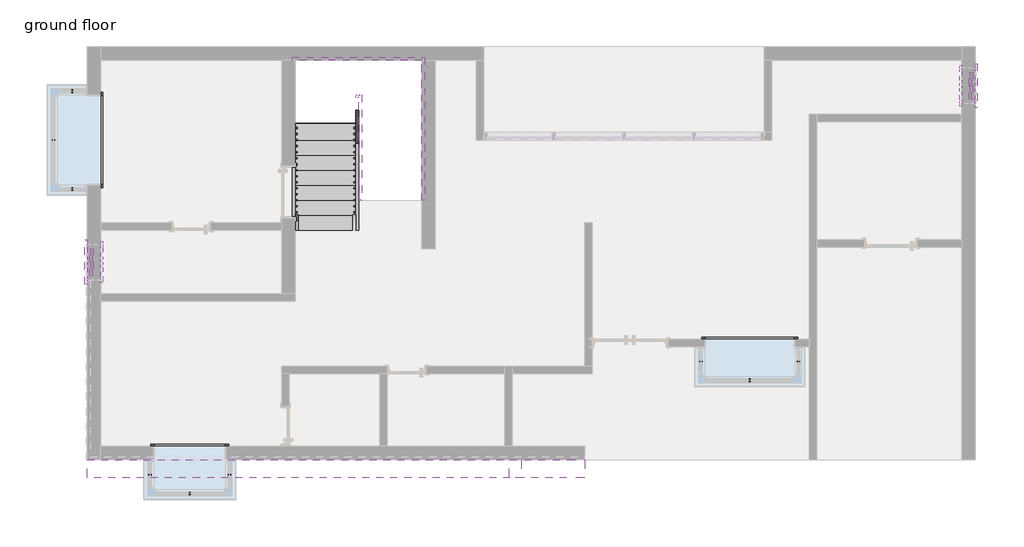
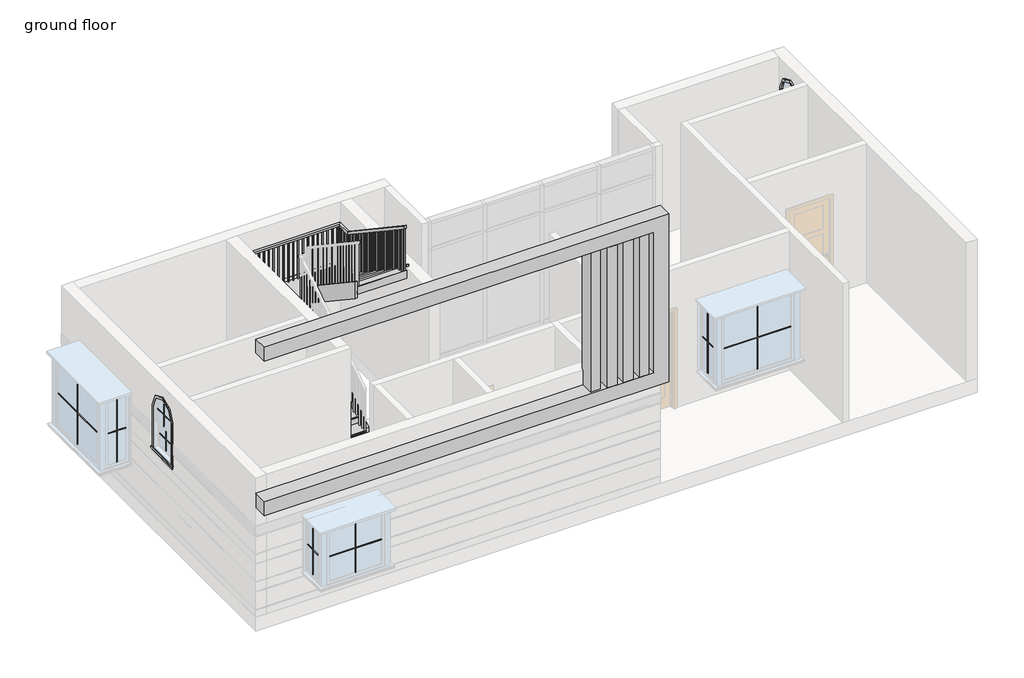
# One storey, part 5 of 5: 22 proxies, 6 members, 1 railing, 1 stair flight.
"""IFC4 building model written with IfcOpenShell, lengths in millimetres."""

from ifc_helpers import new_model, si_unit, frame, origin, place, context, project, spatial, polyline, outline, extrude, faceted_brep, transform, mapped, element, save
from components import generic_models_1_generic_models_1_e2d67b9d, generic_models_2_generic_models_2_13199aed, muntin_pattern_2x2_muntin_pattern_2x2_eeef18e2, muntin_pattern_2x2_muntin_pattern_2x2_218eda85, muntin_pattern_2x2_muntin_pattern_2x2_3440c8d2, muntin_pattern_2x2_muntin_pattern_2x2_8235f178, muntin_pattern_2x2_muntin_pattern_2x2_f03ab90d, trim_window_exterior_arch_hung_with_sill_ae9dfc94, trim_window_interior_arch_hung_picture_frame_76300bdb, trim_window_interior_flat_picture_frame_524b5c54, trim_window_interior_flat_picture_frame_ace0ae79, stair_flight_95751e6d

model = new_model("IFC4")

# Units and contexts
model_context = context("Model", 3, world=origin())
ifc_project = project(units=[si_unit("LENGTHUNIT", "METRE", prefix="MILLI")], contexts=[model_context])

# Site, building, storey
site = spatial("IfcSite", under=ifc_project)
building = spatial("IfcBuilding", under=site)
storey = spatial("IfcBuildingStorey", under=building, Name="ground floor", Elevation=304.8)

# Proxies
placement = place(None, origin())
generic_models_1_generic_models_1_shape = generic_models_1_generic_models_1_e2d67b9d(model_context)
element("IfcBuildingElementProxy", 1, Name="Generic Models 1 : Generic Models 1", ObjectType="Generic Models 1 : Generic Models 1", at=placement, inside=storey, context=model_context, shape_type="MappedRepresentation", body=[
    mapped(generic_models_1_generic_models_1_shape, transform((0.0, 0.0, 0.0), x_axis=(1.0, 0.0, 0.0), y_axis=(0.0, 1.0, 0.0), z_axis=(0.0, 0.0, 1.0))),
])
generic_models_2_generic_models_2_shape = generic_models_2_generic_models_2_13199aed(model_context)
element("IfcBuildingElementProxy", 2, Name="Generic Models 2 : Generic Models 2", ObjectType="Generic Models 2 : Generic Models 2", at=placement, inside=storey, context=model_context, shape_type="MappedRepresentation", body=[
    mapped(generic_models_2_generic_models_2_shape, transform((0.0, 0.0, 0.0), x_axis=(1.0, 0.0, 0.0), y_axis=(0.0, 1.0, 0.0), z_axis=(0.0, 0.0, 1.0))),
])
muntin_pattern_2x2_muntin_pattern_2x2_shape = muntin_pattern_2x2_muntin_pattern_2x2_eeef18e2(model_context)
element("IfcBuildingElementProxy", 3, Name="Muntin Pattern_2x2 : Muntin Pattern_2x2", ObjectType="Muntin Pattern_2x2 : Muntin Pattern_2x2", at=placement, inside=storey, context=model_context, shape_type="MappedRepresentation", body=[
    mapped(muntin_pattern_2x2_muntin_pattern_2x2_shape, transform((-2015.7672301, -5928.5552427, 1035.05), x_axis=(-1.0, 0.0, 0.0), y_axis=(0.0, -1.0, 0.0), z_axis=(0.0, 0.0, 1.0))),
])
element("IfcBuildingElementProxy", 4, Name="Muntin Pattern_2x2 : Muntin Pattern_2x2", ObjectType="Muntin Pattern_2x2 : Muntin Pattern_2x2", at=placement, inside=storey, context=model_context, shape_type="MappedRepresentation", body=[
    mapped(muntin_pattern_2x2_muntin_pattern_2x2_shape, transform((-13747.3922301, -1880.4302427, 1035.05), x_axis=(0.0, 1.0, 0.0), y_axis=(-1.0, 0.0, 0.0), z_axis=(0.0, 0.0, 1.0))),
])
muntin_pattern_2x2_muntin_pattern_2x2_2_shape = muntin_pattern_2x2_muntin_pattern_2x2_218eda85(model_context)
element("IfcBuildingElementProxy", 5, Name="Muntin Pattern_2x2 : Muntin Pattern_2x2", ObjectType="Muntin Pattern_2x2 : Muntin Pattern_2x2", at=placement, inside=storey, context=model_context, shape_type="MappedRepresentation", body=[
    mapped(muntin_pattern_2x2_muntin_pattern_2x2_2_shape, transform((-1193.4422301, -5614.2302427, 1035.05), x_axis=(0.0, 1.0, 0.0), y_axis=(-1.0, 0.0, 0.0), z_axis=(0.0, 0.0, 1.0))),
])
element("IfcBuildingElementProxy", 6, Name="Muntin Pattern_2x2 : Muntin Pattern_2x2", ObjectType="Muntin Pattern_2x2 : Muntin Pattern_2x2", at=placement, inside=storey, context=model_context, shape_type="MappedRepresentation", body=[
    mapped(muntin_pattern_2x2_muntin_pattern_2x2_2_shape, transform((-2838.0922301, -5614.2302427, 1035.05), x_axis=(0.0, -1.0, 0.0), y_axis=(1.0, 0.0, 0.0), z_axis=(0.0, 0.0, 1.0))),
])
element("IfcBuildingElementProxy", 7, Name="Muntin Pattern_2x2 : Muntin Pattern_2x2", ObjectType="Muntin Pattern_2x2 : Muntin Pattern_2x2", at=placement, inside=storey, context=model_context, shape_type="MappedRepresentation", body=[
    mapped(muntin_pattern_2x2_muntin_pattern_2x2_2_shape, transform((-13433.0672301, -2702.7552427, 1035.05), x_axis=(1.0, 0.0, 0.0), y_axis=(0.0, 1.0, 0.0), z_axis=(0.0, 0.0, 1.0))),
])
element("IfcBuildingElementProxy", 8, Name="Muntin Pattern_2x2 : Muntin Pattern_2x2", ObjectType="Muntin Pattern_2x2 : Muntin Pattern_2x2", at=placement, inside=storey, context=model_context, shape_type="MappedRepresentation", body=[
    mapped(muntin_pattern_2x2_muntin_pattern_2x2_2_shape, transform((-13433.0672301, -1058.1052427, 1035.05), x_axis=(-1.0, 0.0, 0.0), y_axis=(0.0, -1.0, 0.0), z_axis=(0.0, 0.0, 1.0))),
])
muntin_pattern_2x2_muntin_pattern_2x2_3_shape = muntin_pattern_2x2_muntin_pattern_2x2_3440c8d2(model_context)
element("IfcBuildingElementProxy", 9, Name="Muntin Pattern_2x2 : Muntin Pattern_2x2", ObjectType="Muntin Pattern_2x2 : Muntin Pattern_2x2", at=placement, inside=storey, context=model_context, shape_type="MappedRepresentation", body=[
    mapped(muntin_pattern_2x2_muntin_pattern_2x2_3_shape, transform((-13144.1422301, -3937.8302427, 2460.625), x_axis=(0.0, 1.0, 0.0), y_axis=(-1.0, 0.0, 0.0), z_axis=(0.0, 0.0, 1.0))),
])
element("IfcBuildingElementProxy", 10, Name="Muntin Pattern_2x2 : Muntin Pattern_2x2", ObjectType="Muntin Pattern_2x2 : Muntin Pattern_2x2", at=placement, inside=storey, context=model_context, shape_type="MappedRepresentation", body=[
    mapped(muntin_pattern_2x2_muntin_pattern_2x2_3_shape, transform((-13099.6922301, -3937.8302427, 1905.0), x_axis=(0.0, 1.0, 0.0), y_axis=(-1.0, 0.0, 0.0), z_axis=(0.0, 0.0, 1.0))),
])
element("IfcBuildingElementProxy", 11, Name="Muntin Pattern_2x2 : Muntin Pattern_2x2", ObjectType="Muntin Pattern_2x2 : Muntin Pattern_2x2", at=placement, inside=storey, context=model_context, shape_type="MappedRepresentation", body=[
    mapped(muntin_pattern_2x2_muntin_pattern_2x2_3_shape, transform((1746.6077699, -966.0302427, 2460.625), x_axis=(0.0, -1.0, 0.0), y_axis=(1.0, 0.0, 0.0), z_axis=(0.0, 0.0, 1.0))),
])
element("IfcBuildingElementProxy", 12, Name="Muntin Pattern_2x2 : Muntin Pattern_2x2", ObjectType="Muntin Pattern_2x2 : Muntin Pattern_2x2", at=placement, inside=storey, context=model_context, shape_type="MappedRepresentation", body=[
    mapped(muntin_pattern_2x2_muntin_pattern_2x2_3_shape, transform((1702.1577699, -966.0302427, 1905.0), x_axis=(0.0, -1.0, 0.0), y_axis=(1.0, 0.0, 0.0), z_axis=(0.0, 0.0, 1.0))),
])
muntin_pattern_2x2_muntin_pattern_2x2_4_shape = muntin_pattern_2x2_muntin_pattern_2x2_8235f178(model_context)
element("IfcBuildingElementProxy", 13, Name="Muntin Pattern_2x2 : Muntin Pattern_2x2", ObjectType="Muntin Pattern_2x2 : Muntin Pattern_2x2", at=placement, inside=storey, context=model_context, shape_type="MappedRepresentation", body=[
    mapped(muntin_pattern_2x2_muntin_pattern_2x2_4_shape, transform((-11451.8672301, -7833.5552427, 1035.05), x_axis=(-1.0, 0.0, 0.0), y_axis=(0.0, -1.0, 0.0), z_axis=(0.0, 0.0, 1.0))),
])
muntin_pattern_2x2_muntin_pattern_2x2_5_shape = muntin_pattern_2x2_muntin_pattern_2x2_f03ab90d(model_context)
element("IfcBuildingElementProxy", 14, Name="Muntin Pattern_2x2 : Muntin Pattern_2x2", ObjectType="Muntin Pattern_2x2 : Muntin Pattern_2x2", at=placement, inside=storey, context=model_context, shape_type="MappedRepresentation", body=[
    mapped(muntin_pattern_2x2_muntin_pattern_2x2_5_shape, transform((-10781.9422301, -7519.2302427, 1035.05), x_axis=(0.0, 1.0, 0.0), y_axis=(-1.0, 0.0, 0.0), z_axis=(0.0, 0.0, 1.0))),
])
element("IfcBuildingElementProxy", 15, Name="Muntin Pattern_2x2 : Muntin Pattern_2x2", ObjectType="Muntin Pattern_2x2 : Muntin Pattern_2x2", at=placement, inside=storey, context=model_context, shape_type="MappedRepresentation", body=[
    mapped(muntin_pattern_2x2_muntin_pattern_2x2_5_shape, transform((-12121.7922301, -7519.2302427, 1035.05), x_axis=(0.0, -1.0, 0.0), y_axis=(1.0, 0.0, 0.0), z_axis=(0.0, 0.0, 1.0))),
])
trim_window_exterior_arch_hung_with_sill_shape = trim_window_exterior_arch_hung_with_sill_ae9dfc94(model_context)
element("IfcBuildingElementProxy", 16, Name="Trim-Window-Exterior-Arch-Hung : with Sill", ObjectType="Trim-Window-Exterior-Arch-Hung : with Sill", at=placement, inside=storey, context=model_context, shape_type="MappedRepresentation", body=[
    mapped(trim_window_exterior_arch_hung_with_sill_shape, transform((-13179.0672301, -3937.8302427, 3048.0), x_axis=(0.0, -1.0, 0.0), y_axis=(0.0, 0.0, 1.0), z_axis=(-1.0, 0.0, 0.0))),
])
element("IfcBuildingElementProxy", 17, Name="Trim-Window-Exterior-Arch-Hung : with Sill", ObjectType="Trim-Window-Exterior-Arch-Hung : with Sill", at=placement, inside=storey, context=model_context, shape_type="MappedRepresentation", body=[
    mapped(trim_window_exterior_arch_hung_with_sill_shape, transform((1781.5327699, -966.0302427, 3048.0), x_axis=(0.0, 1.0, 0.0), y_axis=(0.0, 0.0, 1.0), z_axis=(1.0, 0.0, 0.0))),
])
trim_window_interior_arch_hung_picture_frame_shape = trim_window_interior_arch_hung_picture_frame_76300bdb(model_context)
element("IfcBuildingElementProxy", 18, Name="Trim-Window-Interior-Arch-Hung : Picture Frame", ObjectType="Trim-Window-Interior-Arch-Hung : Picture Frame", at=placement, inside=storey, context=model_context, shape_type="MappedRepresentation", body=[
    mapped(trim_window_interior_arch_hung_picture_frame_shape, transform((-12950.4672301, -3937.8302427, 3048.0), x_axis=(0.0, 1.0, 0.0), y_axis=(0.0, 0.0, 1.0), z_axis=(1.0, 0.0, 0.0))),
])
element("IfcBuildingElementProxy", 19, Name="Trim-Window-Interior-Arch-Hung : Picture Frame", ObjectType="Trim-Window-Interior-Arch-Hung : Picture Frame", at=placement, inside=storey, context=model_context, shape_type="MappedRepresentation", body=[
    mapped(trim_window_interior_arch_hung_picture_frame_shape, transform((1552.9327699, -966.0302427, 3048.0), x_axis=(0.0, -1.0, 0.0), y_axis=(0.0, 0.0, 1.0), z_axis=(-1.0, 0.0, 0.0))),
])
trim_window_interior_flat_picture_frame_shape = trim_window_interior_flat_picture_frame_524b5c54(model_context)
element("IfcBuildingElementProxy", 20, Name="Trim-Window-Interior-Flat : Picture Frame", ObjectType="Trim-Window-Interior-Flat : Picture Frame", at=placement, inside=storey, context=model_context, shape_type="MappedRepresentation", body=[
    mapped(trim_window_interior_flat_picture_frame_shape, transform((-2015.7672301, -5233.2302427, 2489.2), x_axis=(-1.0, 0.0, 0.0), y_axis=(0.0, 0.0, 1.0), z_axis=(0.0, 1.0, 0.0))),
])
element("IfcBuildingElementProxy", 21, Name="Trim-Window-Interior-Flat : Picture Frame", ObjectType="Trim-Window-Interior-Flat : Picture Frame", at=placement, inside=storey, context=model_context, shape_type="MappedRepresentation", body=[
    mapped(trim_window_interior_flat_picture_frame_shape, transform((-12950.4672301, -1880.4302427, 2489.2), x_axis=(0.0, 1.0, 0.0), y_axis=(0.0, 0.0, 1.0), z_axis=(1.0, 0.0, 0.0))),
])
trim_window_interior_flat_picture_frame_2_shape = trim_window_interior_flat_picture_frame_ace0ae79(model_context)
element("IfcBuildingElementProxy", 22, Name="Trim-Window-Interior-Flat : Picture Frame", ObjectType="Trim-Window-Interior-Flat : Picture Frame", at=placement, inside=storey, context=model_context, shape_type="MappedRepresentation", body=[
    mapped(trim_window_interior_flat_picture_frame_2_shape, transform((-11451.8672301, -7036.6302427, 2184.4), x_axis=(-1.0, 0.0, 0.0), y_axis=(0.0, 0.0, 1.0), z_axis=(0.0, 1.0, 0.0))),
])

# Members
element("IfcMember", 23, ObjectType="Stringer - 2\" Width", at=placement, inside=storey, context=model_context, shape_type="SweptSolid", body=[
    extrude(outline(polyline([(-3404.4302427, 304.8), (-3404.4302427, 522.8398409), (-1077.1900041, 2074.3333333), (-534.2302427, 2074.3333333), (-534.2302427, 2069.982498), (-3182.0039897, 304.8), (-3404.4302427, 304.8)])), frame((-9724.6672301, 0.0, 0.0), z_axis=(1.0, 0.0, 0.0), x_axis=(0.0, 1.0, 0.0)), (0.0, 0.0, 1.0), 50.8),
])
element("IfcMember", 24, ObjectType="Stringer - 2\" Width", at=placement, inside=storey, context=model_context, shape_type="SweptSolid", body=[
    extrude(outline(polyline([(-9724.6672301, -534.2302427), (-9724.6672301, -483.4302427), (-7540.2672301, -483.4302427), (-7540.2672301, -534.2302427), (-9724.6672301, -534.2302427)])), frame((0.0, 0.0, 1769.5333333), z_axis=(0.0, 0.0, 1.0), x_axis=(1.0, 0.0, 0.0)), (0.0, 0.0, 1.0), 304.8),
])
element("IfcMember", 25, ObjectType="Stringer - 2\" Width", at=placement, inside=storey, context=model_context, shape_type="SweptSolid", body=[
    extrude(outline(polyline([(-483.4302427, 1792.8398409), (-483.4302427, 1769.5333333), (-997.9564957, 1769.5333333), (-2896.4302427, 3035.182498), (-2896.4302427, 3401.5065076), (-483.4302427, 1792.8398409)])), frame((-7540.2672301, 0.0, 0.0), z_axis=(1.0, 0.0, 0.0), x_axis=(0.0, 1.0, 0.0)), (0.0, 0.0, 1.0), 50.8),
])
element("IfcMember", 26, ObjectType="Stringer - 2\" Width", at=placement, inside=storey, context=model_context, shape_type="SweptSolid", body=[
    extrude(outline(polyline([(-3404.4302427, 304.8), (-3404.4302427, 522.8398409), (-1169.2302427, 2012.9731743), (-1169.2302427, 1646.6491647), (-3182.0039897, 304.8), (-3404.4302427, 304.8)])), frame((-8657.8672301, 0.0, 0.0), z_axis=(1.0, 0.0, 0.0), x_axis=(0.0, 1.0, 0.0)), (0.0, 0.0, 1.0), 50.8),
])
element("IfcMember", 27, ObjectType="Stringer - 2\" Width", at=placement, inside=storey, context=model_context, shape_type="SweptSolid", body=[
    extrude(outline(polyline([(-8657.8672301, -1169.2302427), (-8657.8672301, -1118.4302427), (-8607.0672301, -1118.4302427), (-8607.0672301, -1169.2302427), (-8657.8672301, -1169.2302427)])), frame((0.0, 0.0, 1769.5333333), z_axis=(0.0, 0.0, 1.0), x_axis=(1.0, 0.0, 0.0)), (0.0, 0.0, 1.0), 304.8),
])
element("IfcMember", 28, ObjectType="Stringer - 2\" Width", at=placement, inside=storey, context=model_context, shape_type="SweptSolid", body=[
    extrude(outline(polyline([(-1118.4302427, 2216.1731743), (-1118.4302427, 1849.8491647), (-2896.4302427, 3035.182498), (-2896.4302427, 3401.5065076), (-1118.4302427, 2216.1731743)])), frame((-8607.0672301, 0.0, 0.0), z_axis=(1.0, 0.0, 0.0), x_axis=(0.0, 1.0, 0.0)), (0.0, 0.0, 1.0), 50.8),
])

# Railing
element("IfcRailing", 29, ObjectType="Handrail - Rectangular", at=placement, inside=storey, context=model_context, shape_type="SolidModel", body=[
    faceted_brep([(-9673.8672301, -3404.4302427, 1388.5333333), (-9673.8672301, -3404.4302427, 1327.4793317), (-9623.0672301, -3404.4302427, 1327.4793317), (-9623.0672301, -3404.4302427, 1388.5333333), (-9673.8672301, -1118.4302427, 2912.5333333), (-9673.8672301, -1103.0492403, 2861.7333333), (-9623.0672301, -1103.0492403, 2861.7333333), (-9623.0672301, -1118.4302427, 2912.5333333), (-9673.8672301, -534.2302427, 2912.5333333), (-9673.8672301, -534.2302427, 2861.7333333), (-9623.0672301, -585.0302427, 2861.7333333), (-9623.0672301, -585.0302427, 2912.5333333), (-7540.2672301, -534.2302427, 2912.5333333), (-7540.2672301, -534.2302427, 2861.7333333), (-7591.0672301, -585.0302427, 2861.7333333), (-7591.0672301, -585.0302427, 2912.5333333), (-7540.2672301, -864.4302427, 2912.5333333), (-7540.2672301, -879.8112451, 2861.7333333), (-7591.0672301, -879.8112451, 2861.7333333), (-7591.0672301, -864.4302427, 2912.5333333), (-7540.2672301, -2896.4302427, 4267.2), (-7591.0672301, -2896.4302427, 4267.2), (-7591.0672301, -2896.4302427, 4206.1459984), (-7540.2672301, -2896.4302427, 4206.1459984)], [[[0, 1, 2, 3]], [[1, 0, 4, 5]], [[2, 1, 5, 6]], [[3, 2, 6, 7]], [[0, 3, 7, 4]], [[5, 4, 8, 9]], [[6, 5, 9, 10]], [[7, 6, 10, 11]], [[4, 7, 11, 8]], [[9, 8, 12, 13]], [[10, 9, 13, 14]], [[11, 10, 14, 15]], [[8, 11, 15, 12]], [[13, 12, 16, 17]], [[14, 13, 17, 18]], [[15, 14, 18, 19]], [[12, 15, 19, 16]], [[20, 21, 22, 23]], [[17, 16, 20, 23]], [[18, 17, 23, 22]], [[19, 18, 22, 21]], [[16, 19, 21, 20]]]),
    extrude(outline(polyline([(-2785.3052427, 4132.0626651), (-2785.3052427, 3183.4666667), (-2804.3552427, 3183.4666667), (-2804.3552427, 4144.7626651), (-2785.3052427, 4132.0626651)])), frame((-7575.1922301, 0.0, 0.0), z_axis=(1.0, 0.0, 0.0), x_axis=(0.0, 1.0, 0.0)), (0.0, 0.0, 1.0), 19.05),
    extrude(outline(polyline([(-2683.7052427, 4064.3293317), (-2683.7052427, 3183.4666667), (-2702.7552427, 3183.4666667), (-2702.7552427, 4077.0293317), (-2683.7052427, 4064.3293317)])), frame((-7575.1922301, 0.0, 0.0), z_axis=(1.0, 0.0, 0.0), x_axis=(0.0, 1.0, 0.0)), (0.0, 0.0, 1.0), 19.05),
    extrude(outline(polyline([(-2582.1052427, 3996.5959984), (-2582.1052427, 3014.1333333), (-2601.1552427, 3014.1333333), (-2601.1552427, 4009.2959984), (-2582.1052427, 3996.5959984)])), frame((-7575.1922301, 0.0, 0.0), z_axis=(1.0, 0.0, 0.0), x_axis=(0.0, 1.0, 0.0)), (0.0, 0.0, 1.0), 19.05),
    extrude(outline(polyline([(-2480.5052427, 3928.8626651), (-2480.5052427, 3014.1333333), (-2499.5552427, 3014.1333333), (-2499.5552427, 3941.5626651), (-2480.5052427, 3928.8626651)])), frame((-7575.1922301, 0.0, 0.0), z_axis=(1.0, 0.0, 0.0), x_axis=(0.0, 1.0, 0.0)), (0.0, 0.0, 1.0), 19.05),
    extrude(outline(polyline([(-2378.9052427, 3861.1293317), (-2378.9052427, 3014.1333333), (-2397.9552427, 3014.1333333), (-2397.9552427, 3873.8293317), (-2378.9052427, 3861.1293317)])), frame((-7575.1922301, 0.0, 0.0), z_axis=(1.0, 0.0, 0.0), x_axis=(0.0, 1.0, 0.0)), (0.0, 0.0, 1.0), 19.05),
    extrude(outline(polyline([(-2277.3052427, 3793.3959984), (-2277.3052427, 2844.8), (-2296.3552427, 2844.8), (-2296.3552427, 3806.0959984), (-2277.3052427, 3793.3959984)])), frame((-7575.1922301, 0.0, 0.0), z_axis=(1.0, 0.0, 0.0), x_axis=(0.0, 1.0, 0.0)), (0.0, 0.0, 1.0), 19.05),
    extrude(outline(polyline([(-2175.7052427, 3725.6626651), (-2175.7052427, 2844.8), (-2194.7552427, 2844.8), (-2194.7552427, 3738.3626651), (-2175.7052427, 3725.6626651)])), frame((-7575.1922301, 0.0, 0.0), z_axis=(1.0, 0.0, 0.0), x_axis=(0.0, 1.0, 0.0)), (0.0, 0.0, 1.0), 19.05),
    extrude(outline(polyline([(-2074.1052427, 3657.9293317), (-2074.1052427, 2675.4666667), (-2093.1552427, 2675.4666667), (-2093.1552427, 3670.6293317), (-2074.1052427, 3657.9293317)])), frame((-7575.1922301, 0.0, 0.0), z_axis=(1.0, 0.0, 0.0), x_axis=(0.0, 1.0, 0.0)), (0.0, 0.0, 1.0), 19.05),
    extrude(outline(polyline([(-1972.5052427, 3590.1959984), (-1972.5052427, 2675.4666667), (-1991.5552427, 2675.4666667), (-1991.5552427, 3602.8959984), (-1972.5052427, 3590.1959984)])), frame((-7575.1922301, 0.0, 0.0), z_axis=(1.0, 0.0, 0.0), x_axis=(0.0, 1.0, 0.0)), (0.0, 0.0, 1.0), 19.05),
    extrude(outline(polyline([(-1870.9052427, 3522.4626651), (-1870.9052427, 2675.4666667), (-1889.9552427, 2675.4666667), (-1889.9552427, 3535.1626651), (-1870.9052427, 3522.4626651)])), frame((-7575.1922301, 0.0, 0.0), z_axis=(1.0, 0.0, 0.0), x_axis=(0.0, 1.0, 0.0)), (0.0, 0.0, 1.0), 19.05),
    extrude(outline(polyline([(-1769.3052427, 3454.7293317), (-1769.3052427, 2506.1333333), (-1788.3552427, 2506.1333333), (-1788.3552427, 3467.4293317), (-1769.3052427, 3454.7293317)])), frame((-7575.1922301, 0.0, 0.0), z_axis=(1.0, 0.0, 0.0), x_axis=(0.0, 1.0, 0.0)), (0.0, 0.0, 1.0), 19.05),
    extrude(outline(polyline([(-1667.7052427, 3386.9959984), (-1667.7052427, 2506.1333333), (-1686.7552427, 2506.1333333), (-1686.7552427, 3399.6959984), (-1667.7052427, 3386.9959984)])), frame((-7575.1922301, 0.0, 0.0), z_axis=(1.0, 0.0, 0.0), x_axis=(0.0, 1.0, 0.0)), (0.0, 0.0, 1.0), 19.05),
    extrude(outline(polyline([(-1566.1052427, 3319.2626651), (-1566.1052427, 2336.8), (-1585.1552427, 2336.8), (-1585.1552427, 3331.9626651), (-1566.1052427, 3319.2626651)])), frame((-7575.1922301, 0.0, 0.0), z_axis=(1.0, 0.0, 0.0), x_axis=(0.0, 1.0, 0.0)), (0.0, 0.0, 1.0), 19.05),
    extrude(outline(polyline([(-1464.5052427, 3251.5293317), (-1464.5052427, 2336.8), (-1483.5552427, 2336.8), (-1483.5552427, 3264.2293317), (-1464.5052427, 3251.5293317)])), frame((-7575.1922301, 0.0, 0.0), z_axis=(1.0, 0.0, 0.0), x_axis=(0.0, 1.0, 0.0)), (0.0, 0.0, 1.0), 19.05),
    extrude(outline(polyline([(-1362.9052427, 3183.7959984), (-1362.9052427, 2336.8), (-1381.9552427, 2336.8), (-1381.9552427, 3196.4959984), (-1362.9052427, 3183.7959984)])), frame((-7575.1922301, 0.0, 0.0), z_axis=(1.0, 0.0, 0.0), x_axis=(0.0, 1.0, 0.0)), (0.0, 0.0, 1.0), 19.05),
    extrude(outline(polyline([(-1261.3052427, 3116.0626651), (-1261.3052427, 2167.4666667), (-1280.3552427, 2167.4666667), (-1280.3552427, 3128.7626651), (-1261.3052427, 3116.0626651)])), frame((-7575.1922301, 0.0, 0.0), z_axis=(1.0, 0.0, 0.0), x_axis=(0.0, 1.0, 0.0)), (0.0, 0.0, 1.0), 19.05),
    extrude(outline(polyline([(-1159.7052427, 3048.3293317), (-1159.7052427, 2167.4666667), (-1178.7552427, 2167.4666667), (-1178.7552427, 3061.0293317), (-1159.7052427, 3048.3293317)])), frame((-7575.1922301, 0.0, 0.0), z_axis=(1.0, 0.0, 0.0), x_axis=(0.0, 1.0, 0.0)), (0.0, 0.0, 1.0), 19.05),
    extrude(outline(polyline([(-1058.1052427, 2980.5959984), (-1058.1052427, 1998.1333333), (-1077.1552427, 1998.1333333), (-1077.1552427, 2993.2959984), (-1058.1052427, 2980.5959984)])), frame((-7575.1922301, 0.0, 0.0), z_axis=(1.0, 0.0, 0.0), x_axis=(0.0, 1.0, 0.0)), (0.0, 0.0, 1.0), 19.05),
    extrude(outline(polyline([(-956.5052427, 2912.8626651), (-956.5052427, 1998.1333333), (-975.5552427, 1998.1333333), (-975.5552427, 2925.5626651), (-956.5052427, 2912.8626651)])), frame((-7575.1922301, 0.0, 0.0), z_axis=(1.0, 0.0, 0.0), x_axis=(0.0, 1.0, 0.0)), (0.0, 0.0, 1.0), 19.05),
    extrude(outline(polyline([(-7556.1422301, -854.9052427), (-7556.1422301, -873.9552427), (-7575.1922301, -873.9552427), (-7575.1922301, -854.9052427), (-7556.1422301, -854.9052427)])), frame((0.0, 0.0, 1998.1333333), z_axis=(0.0, 0.0, 1.0), x_axis=(1.0, 0.0, 0.0)), (0.0, 0.0, 1.0), 863.6),
    extrude(outline(polyline([(-7556.1422301, -753.3052427), (-7556.1422301, -772.3552427), (-7575.1922301, -772.3552427), (-7575.1922301, -753.3052427), (-7556.1422301, -753.3052427)])), frame((0.0, 0.0, 1998.1333333), z_axis=(0.0, 0.0, 1.0), x_axis=(1.0, 0.0, 0.0)), (0.0, 0.0, 1.0), 863.6),
    extrude(outline(polyline([(-7556.1422301, -651.7052427), (-7556.1422301, -670.7552427), (-7575.1922301, -670.7552427), (-7575.1922301, -651.7052427), (-7556.1422301, -651.7052427)])), frame((0.0, 0.0, 1998.1333333), z_axis=(0.0, 0.0, 1.0), x_axis=(1.0, 0.0, 0.0)), (0.0, 0.0, 1.0), 863.6),
    extrude(outline(polyline([(-7625.9922301, -550.1052427), (-7606.9422301, -550.1052427), (-7606.9422301, -569.1552427), (-7625.9922301, -569.1552427), (-7625.9922301, -550.1052427)])), frame((0.0, 0.0, 1998.1333333), z_axis=(0.0, 0.0, 1.0), x_axis=(1.0, 0.0, 0.0)), (0.0, 0.0, 1.0), 863.6),
    extrude(outline(polyline([(-7727.5922301, -550.1052427), (-7708.5422301, -550.1052427), (-7708.5422301, -569.1552427), (-7727.5922301, -569.1552427), (-7727.5922301, -550.1052427)])), frame((0.0, 0.0, 1998.1333333), z_axis=(0.0, 0.0, 1.0), x_axis=(1.0, 0.0, 0.0)), (0.0, 0.0, 1.0), 863.6),
    extrude(outline(polyline([(-7829.1922301, -550.1052427), (-7810.1422301, -550.1052427), (-7810.1422301, -569.1552427), (-7829.1922301, -569.1552427), (-7829.1922301, -550.1052427)])), frame((0.0, 0.0, 1998.1333333), z_axis=(0.0, 0.0, 1.0), x_axis=(1.0, 0.0, 0.0)), (0.0, 0.0, 1.0), 863.6),
    extrude(outline(polyline([(-7930.7922301, -550.1052427), (-7911.7422301, -550.1052427), (-7911.7422301, -569.1552427), (-7930.7922301, -569.1552427), (-7930.7922301, -550.1052427)])), frame((0.0, 0.0, 1998.1333333), z_axis=(0.0, 0.0, 1.0), x_axis=(1.0, 0.0, 0.0)), (0.0, 0.0, 1.0), 863.6),
    extrude(outline(polyline([(-8032.3922301, -550.1052427), (-8013.3422301, -550.1052427), (-8013.3422301, -569.1552427), (-8032.3922301, -569.1552427), (-8032.3922301, -550.1052427)])), frame((0.0, 0.0, 1998.1333333), z_axis=(0.0, 0.0, 1.0), x_axis=(1.0, 0.0, 0.0)), (0.0, 0.0, 1.0), 863.6),
    extrude(outline(polyline([(-8133.9922301, -550.1052427), (-8114.9422301, -550.1052427), (-8114.9422301, -569.1552427), (-8133.9922301, -569.1552427), (-8133.9922301, -550.1052427)])), frame((0.0, 0.0, 1998.1333333), z_axis=(0.0, 0.0, 1.0), x_axis=(1.0, 0.0, 0.0)), (0.0, 0.0, 1.0), 863.6),
    extrude(outline(polyline([(-8235.5922301, -550.1052427), (-8216.5422301, -550.1052427), (-8216.5422301, -569.1552427), (-8235.5922301, -569.1552427), (-8235.5922301, -550.1052427)])), frame((0.0, 0.0, 1998.1333333), z_axis=(0.0, 0.0, 1.0), x_axis=(1.0, 0.0, 0.0)), (0.0, 0.0, 1.0), 863.6),
    extrude(outline(polyline([(-8337.1922301, -550.1052427), (-8318.1422301, -550.1052427), (-8318.1422301, -569.1552427), (-8337.1922301, -569.1552427), (-8337.1922301, -550.1052427)])), frame((0.0, 0.0, 1998.1333333), z_axis=(0.0, 0.0, 1.0), x_axis=(1.0, 0.0, 0.0)), (0.0, 0.0, 1.0), 863.6),
    extrude(outline(polyline([(-8438.7922301, -550.1052427), (-8419.7422301, -550.1052427), (-8419.7422301, -569.1552427), (-8438.7922301, -569.1552427), (-8438.7922301, -550.1052427)])), frame((0.0, 0.0, 1998.1333333), z_axis=(0.0, 0.0, 1.0), x_axis=(1.0, 0.0, 0.0)), (0.0, 0.0, 1.0), 863.6),
    extrude(outline(polyline([(-8540.3922301, -550.1052427), (-8521.3422301, -550.1052427), (-8521.3422301, -569.1552427), (-8540.3922301, -569.1552427), (-8540.3922301, -550.1052427)])), frame((0.0, 0.0, 1998.1333333), z_axis=(0.0, 0.0, 1.0), x_axis=(1.0, 0.0, 0.0)), (0.0, 0.0, 1.0), 863.6),
    extrude(outline(polyline([(-8641.9922301, -550.1052427), (-8622.9422301, -550.1052427), (-8622.9422301, -569.1552427), (-8641.9922301, -569.1552427), (-8641.9922301, -550.1052427)])), frame((0.0, 0.0, 1998.1333333), z_axis=(0.0, 0.0, 1.0), x_axis=(1.0, 0.0, 0.0)), (0.0, 0.0, 1.0), 863.6),
    extrude(outline(polyline([(-8743.5922301, -550.1052427), (-8724.5422301, -550.1052427), (-8724.5422301, -569.1552427), (-8743.5922301, -569.1552427), (-8743.5922301, -550.1052427)])), frame((0.0, 0.0, 1998.1333333), z_axis=(0.0, 0.0, 1.0), x_axis=(1.0, 0.0, 0.0)), (0.0, 0.0, 1.0), 863.6),
    extrude(outline(polyline([(-8845.1922301, -550.1052427), (-8826.1422301, -550.1052427), (-8826.1422301, -569.1552427), (-8845.1922301, -569.1552427), (-8845.1922301, -550.1052427)])), frame((0.0, 0.0, 1998.1333333), z_axis=(0.0, 0.0, 1.0), x_axis=(1.0, 0.0, 0.0)), (0.0, 0.0, 1.0), 863.6),
    extrude(outline(polyline([(-8946.7922301, -550.1052427), (-8927.7422301, -550.1052427), (-8927.7422301, -569.1552427), (-8946.7922301, -569.1552427), (-8946.7922301, -550.1052427)])), frame((0.0, 0.0, 1998.1333333), z_axis=(0.0, 0.0, 1.0), x_axis=(1.0, 0.0, 0.0)), (0.0, 0.0, 1.0), 863.6),
    extrude(outline(polyline([(-9048.3922301, -550.1052427), (-9029.3422301, -550.1052427), (-9029.3422301, -569.1552427), (-9048.3922301, -569.1552427), (-9048.3922301, -550.1052427)])), frame((0.0, 0.0, 1998.1333333), z_axis=(0.0, 0.0, 1.0), x_axis=(1.0, 0.0, 0.0)), (0.0, 0.0, 1.0), 863.6),
    extrude(outline(polyline([(-9149.9922301, -550.1052427), (-9130.9422301, -550.1052427), (-9130.9422301, -569.1552427), (-9149.9922301, -569.1552427), (-9149.9922301, -550.1052427)])), frame((0.0, 0.0, 1998.1333333), z_axis=(0.0, 0.0, 1.0), x_axis=(1.0, 0.0, 0.0)), (0.0, 0.0, 1.0), 863.6),
    extrude(outline(polyline([(-9251.5922301, -550.1052427), (-9232.5422301, -550.1052427), (-9232.5422301, -569.1552427), (-9251.5922301, -569.1552427), (-9251.5922301, -550.1052427)])), frame((0.0, 0.0, 1998.1333333), z_axis=(0.0, 0.0, 1.0), x_axis=(1.0, 0.0, 0.0)), (0.0, 0.0, 1.0), 863.6),
    extrude(outline(polyline([(-9353.1922301, -550.1052427), (-9334.1422301, -550.1052427), (-9334.1422301, -569.1552427), (-9353.1922301, -569.1552427), (-9353.1922301, -550.1052427)])), frame((0.0, 0.0, 1998.1333333), z_axis=(0.0, 0.0, 1.0), x_axis=(1.0, 0.0, 0.0)), (0.0, 0.0, 1.0), 863.6),
    extrude(outline(polyline([(-9454.7922301, -550.1052427), (-9435.7422301, -550.1052427), (-9435.7422301, -569.1552427), (-9454.7922301, -569.1552427), (-9454.7922301, -550.1052427)])), frame((0.0, 0.0, 1998.1333333), z_axis=(0.0, 0.0, 1.0), x_axis=(1.0, 0.0, 0.0)), (0.0, 0.0, 1.0), 863.6),
    extrude(outline(polyline([(-9556.3922301, -550.1052427), (-9537.3422301, -550.1052427), (-9537.3422301, -569.1552427), (-9556.3922301, -569.1552427), (-9556.3922301, -550.1052427)])), frame((0.0, 0.0, 1998.1333333), z_axis=(0.0, 0.0, 1.0), x_axis=(1.0, 0.0, 0.0)), (0.0, 0.0, 1.0), 863.6),
    extrude(outline(polyline([(-9657.9922301, -670.7552427), (-9657.9922301, -651.7052427), (-9638.9422301, -651.7052427), (-9638.9422301, -670.7552427), (-9657.9922301, -670.7552427)])), frame((0.0, 0.0, 1998.1333333), z_axis=(0.0, 0.0, 1.0), x_axis=(1.0, 0.0, 0.0)), (0.0, 0.0, 1.0), 863.6),
    extrude(outline(polyline([(-9657.9922301, -772.3552427), (-9657.9922301, -753.3052427), (-9638.9422301, -753.3052427), (-9638.9422301, -772.3552427), (-9657.9922301, -772.3552427)])), frame((0.0, 0.0, 1998.1333333), z_axis=(0.0, 0.0, 1.0), x_axis=(1.0, 0.0, 0.0)), (0.0, 0.0, 1.0), 863.6),
    extrude(outline(polyline([(-9657.9922301, -873.9552427), (-9657.9922301, -854.9052427), (-9638.9422301, -854.9052427), (-9638.9422301, -873.9552427), (-9657.9922301, -873.9552427)])), frame((0.0, 0.0, 1998.1333333), z_axis=(0.0, 0.0, 1.0), x_axis=(1.0, 0.0, 0.0)), (0.0, 0.0, 1.0), 863.6),
    extrude(outline(polyline([(-9657.9922301, -975.5552427), (-9657.9922301, -956.5052427), (-9638.9422301, -956.5052427), (-9638.9422301, -975.5552427), (-9657.9922301, -975.5552427)])), frame((0.0, 0.0, 1998.1333333), z_axis=(0.0, 0.0, 1.0), x_axis=(1.0, 0.0, 0.0)), (0.0, 0.0, 1.0), 863.6),
    extrude(outline(polyline([(-9657.9922301, -1077.1552427), (-9657.9922301, -1058.1052427), (-9638.9422301, -1058.1052427), (-9638.9422301, -1077.1552427), (-9657.9922301, -1077.1552427)])), frame((0.0, 0.0, 1998.1333333), z_axis=(0.0, 0.0, 1.0), x_axis=(1.0, 0.0, 0.0)), (0.0, 0.0, 1.0), 863.6),
    extrude(outline(polyline([(-1159.7052427, 2823.9626651), (-1159.7052427, 1828.8), (-1178.7552427, 1828.8), (-1178.7552427, 2811.2626651), (-1159.7052427, 2823.9626651)])), frame((-9657.9922301, 0.0, 0.0), z_axis=(1.0, 0.0, 0.0), x_axis=(0.0, 1.0, 0.0)), (0.0, 0.0, 1.0), 19.05),
    extrude(outline(polyline([(-1261.3052427, 2756.2293317), (-1261.3052427, 1828.8), (-1280.3552427, 1828.8), (-1280.3552427, 2743.5293317), (-1261.3052427, 2756.2293317)])), frame((-9657.9922301, 0.0, 0.0), z_axis=(1.0, 0.0, 0.0), x_axis=(0.0, 1.0, 0.0)), (0.0, 0.0, 1.0), 19.05),
    extrude(outline(polyline([(-1362.9052427, 2688.4959984), (-1362.9052427, 1828.8), (-1381.9552427, 1828.8), (-1381.9552427, 2675.7959984), (-1362.9052427, 2688.4959984)])), frame((-9657.9922301, 0.0, 0.0), z_axis=(1.0, 0.0, 0.0), x_axis=(0.0, 1.0, 0.0)), (0.0, 0.0, 1.0), 19.05),
    extrude(outline(polyline([(-1464.5052427, 2620.7626651), (-1464.5052427, 1659.4666667), (-1483.5552427, 1659.4666667), (-1483.5552427, 2608.0626651), (-1464.5052427, 2620.7626651)])), frame((-9657.9922301, 0.0, 0.0), z_axis=(1.0, 0.0, 0.0), x_axis=(0.0, 1.0, 0.0)), (0.0, 0.0, 1.0), 19.05),
    extrude(outline(polyline([(-1566.1052427, 2553.0293317), (-1566.1052427, 1659.4666667), (-1585.1552427, 1659.4666667), (-1585.1552427, 2540.3293317), (-1566.1052427, 2553.0293317)])), frame((-9657.9922301, 0.0, 0.0), z_axis=(1.0, 0.0, 0.0), x_axis=(0.0, 1.0, 0.0)), (0.0, 0.0, 1.0), 19.05),
    extrude(outline(polyline([(-1667.7052427, 2485.2959984), (-1667.7052427, 1490.1333333), (-1686.7552427, 1490.1333333), (-1686.7552427, 2472.5959984), (-1667.7052427, 2485.2959984)])), frame((-9657.9922301, 0.0, 0.0), z_axis=(1.0, 0.0, 0.0), x_axis=(0.0, 1.0, 0.0)), (0.0, 0.0, 1.0), 19.05),
    extrude(outline(polyline([(-1769.3052427, 2417.5626651), (-1769.3052427, 1490.1333333), (-1788.3552427, 1490.1333333), (-1788.3552427, 2404.8626651), (-1769.3052427, 2417.5626651)])), frame((-9657.9922301, 0.0, 0.0), z_axis=(1.0, 0.0, 0.0), x_axis=(0.0, 1.0, 0.0)), (0.0, 0.0, 1.0), 19.05),
    extrude(outline(polyline([(-1870.9052427, 2349.8293317), (-1870.9052427, 1490.1333333), (-1889.9552427, 1490.1333333), (-1889.9552427, 2337.1293317), (-1870.9052427, 2349.8293317)])), frame((-9657.9922301, 0.0, 0.0), z_axis=(1.0, 0.0, 0.0), x_axis=(0.0, 1.0, 0.0)), (0.0, 0.0, 1.0), 19.05),
    extrude(outline(polyline([(-1972.5052427, 2282.0959984), (-1972.5052427, 1320.8), (-1991.5552427, 1320.8), (-1991.5552427, 2269.3959984), (-1972.5052427, 2282.0959984)])), frame((-9657.9922301, 0.0, 0.0), z_axis=(1.0, 0.0, 0.0), x_axis=(0.0, 1.0, 0.0)), (0.0, 0.0, 1.0), 19.05),
    extrude(outline(polyline([(-2074.1052427, 2214.3626651), (-2074.1052427, 1320.8), (-2093.1552427, 1320.8), (-2093.1552427, 2201.6626651), (-2074.1052427, 2214.3626651)])), frame((-9657.9922301, 0.0, 0.0), z_axis=(1.0, 0.0, 0.0), x_axis=(0.0, 1.0, 0.0)), (0.0, 0.0, 1.0), 19.05),
    extrude(outline(polyline([(-2175.7052427, 2146.6293317), (-2175.7052427, 1151.4666667), (-2194.7552427, 1151.4666667), (-2194.7552427, 2133.9293317), (-2175.7052427, 2146.6293317)])), frame((-9657.9922301, 0.0, 0.0), z_axis=(1.0, 0.0, 0.0), x_axis=(0.0, 1.0, 0.0)), (0.0, 0.0, 1.0), 19.05),
    extrude(outline(polyline([(-2277.3052427, 2078.8959984), (-2277.3052427, 1151.4666667), (-2296.3552427, 1151.4666667), (-2296.3552427, 2066.1959984), (-2277.3052427, 2078.8959984)])), frame((-9657.9922301, 0.0, 0.0), z_axis=(1.0, 0.0, 0.0), x_axis=(0.0, 1.0, 0.0)), (0.0, 0.0, 1.0), 19.05),
    extrude(outline(polyline([(-2378.9052427, 2011.1626651), (-2378.9052427, 1151.4666667), (-2397.9552427, 1151.4666667), (-2397.9552427, 1998.4626651), (-2378.9052427, 2011.1626651)])), frame((-9657.9922301, 0.0, 0.0), z_axis=(1.0, 0.0, 0.0), x_axis=(0.0, 1.0, 0.0)), (0.0, 0.0, 1.0), 19.05),
    extrude(outline(polyline([(-2480.5052427, 1943.4293317), (-2480.5052427, 982.1333333), (-2499.5552427, 982.1333333), (-2499.5552427, 1930.7293317), (-2480.5052427, 1943.4293317)])), frame((-9657.9922301, 0.0, 0.0), z_axis=(1.0, 0.0, 0.0), x_axis=(0.0, 1.0, 0.0)), (0.0, 0.0, 1.0), 19.05),
    extrude(outline(polyline([(-2582.1052427, 1875.6959984), (-2582.1052427, 982.1333333), (-2601.1552427, 982.1333333), (-2601.1552427, 1862.9959984), (-2582.1052427, 1875.6959984)])), frame((-9657.9922301, 0.0, 0.0), z_axis=(1.0, 0.0, 0.0), x_axis=(0.0, 1.0, 0.0)), (0.0, 0.0, 1.0), 19.05),
    extrude(outline(polyline([(-2683.7052427, 1807.9626651), (-2683.7052427, 812.8), (-2702.7552427, 812.8), (-2702.7552427, 1795.2626651), (-2683.7052427, 1807.9626651)])), frame((-9657.9922301, 0.0, 0.0), z_axis=(1.0, 0.0, 0.0), x_axis=(0.0, 1.0, 0.0)), (0.0, 0.0, 1.0), 19.05),
    extrude(outline(polyline([(-2785.3052427, 1740.2293317), (-2785.3052427, 812.8), (-2804.3552427, 812.8), (-2804.3552427, 1727.5293317), (-2785.3052427, 1740.2293317)])), frame((-9657.9922301, 0.0, 0.0), z_axis=(1.0, 0.0, 0.0), x_axis=(0.0, 1.0, 0.0)), (0.0, 0.0, 1.0), 19.05),
    extrude(outline(polyline([(-2886.9052427, 1672.4959984), (-2886.9052427, 812.8), (-2905.9552427, 812.8), (-2905.9552427, 1659.7959984), (-2886.9052427, 1672.4959984)])), frame((-9657.9922301, 0.0, 0.0), z_axis=(1.0, 0.0, 0.0), x_axis=(0.0, 1.0, 0.0)), (0.0, 0.0, 1.0), 19.05),
    extrude(outline(polyline([(-2988.5052427, 1604.7626651), (-2988.5052427, 643.4666667), (-3007.5552427, 643.4666667), (-3007.5552427, 1592.0626651), (-2988.5052427, 1604.7626651)])), frame((-9657.9922301, 0.0, 0.0), z_axis=(1.0, 0.0, 0.0), x_axis=(0.0, 1.0, 0.0)), (0.0, 0.0, 1.0), 19.05),
    extrude(outline(polyline([(-3090.1052427, 1537.0293317), (-3090.1052427, 643.4666667), (-3109.1552427, 643.4666667), (-3109.1552427, 1524.3293317), (-3090.1052427, 1537.0293317)])), frame((-9657.9922301, 0.0, 0.0), z_axis=(1.0, 0.0, 0.0), x_axis=(0.0, 1.0, 0.0)), (0.0, 0.0, 1.0), 19.05),
    extrude(outline(polyline([(-3191.7052427, 1469.2959984), (-3191.7052427, 474.1333333), (-3210.7552427, 474.1333333), (-3210.7552427, 1456.5959984), (-3191.7052427, 1469.2959984)])), frame((-9657.9922301, 0.0, 0.0), z_axis=(1.0, 0.0, 0.0), x_axis=(0.0, 1.0, 0.0)), (0.0, 0.0, 1.0), 19.05),
    extrude(outline(polyline([(-3293.3052427, 1401.5626651), (-3293.3052427, 474.1333333), (-3312.3552427, 474.1333333), (-3312.3552427, 1388.8626651), (-3293.3052427, 1401.5626651)])), frame((-9657.9922301, 0.0, 0.0), z_axis=(1.0, 0.0, 0.0), x_axis=(0.0, 1.0, 0.0)), (0.0, 0.0, 1.0), 19.05),
    extrude(outline(polyline([(-7575.1922301, -550.1052427), (-7556.1422301, -550.1052427), (-7556.1422301, -569.1552427), (-7575.1922301, -569.1552427), (-7575.1922301, -550.1052427)])), frame((0.0, 0.0, 1998.1333333), z_axis=(0.0, 0.0, 1.0), x_axis=(1.0, 0.0, 0.0)), (0.0, 0.0, 1.0), 863.6),
    extrude(outline(polyline([(-9657.9922301, -569.1552427), (-9657.9922301, -550.1052427), (-9638.9422301, -550.1052427), (-9638.9422301, -569.1552427), (-9657.9922301, -569.1552427)])), frame((0.0, 0.0, 1998.1333333), z_axis=(0.0, 0.0, 1.0), x_axis=(1.0, 0.0, 0.0)), (0.0, 0.0, 1.0), 863.6),
    extrude(outline(polyline([(-2877.3802427, 4193.4459984), (-2877.3802427, 3183.4666667), (-2896.4302427, 3183.4666667), (-2896.4302427, 4206.1459984), (-2877.3802427, 4193.4459984)])), frame((-7575.1922301, 0.0, 0.0), z_axis=(1.0, 0.0, 0.0), x_axis=(0.0, 1.0, 0.0)), (0.0, 0.0, 1.0), 19.05),
    extrude(outline(polyline([(-3385.3802427, 1340.1793317), (-3385.3802427, 474.1333333), (-3404.4302427, 474.1333333), (-3404.4302427, 1327.4793317), (-3385.3802427, 1340.1793317)])), frame((-9657.9922301, 0.0, 0.0), z_axis=(1.0, 0.0, 0.0), x_axis=(0.0, 1.0, 0.0)), (0.0, 0.0, 1.0), 19.05),
])

# Stair flight
stair_flight_shape = stair_flight_95751e6d(model_context)
element("IfcStairFlight", 30, ObjectType="2\" Tread 1\" Nosing 1/4\" Riser", at=placement, inside=storey, context=model_context, shape_type="MappedRepresentation", body=[
    mapped(stair_flight_shape, transform((0.0, 0.0, 0.0), x_axis=(1.0, 0.0, 0.0), y_axis=(0.0, 1.0, 0.0), z_axis=(0.0, 0.0, 1.0))),
])

save(model, "model.ifc")

# Revit data of these elements
# Type "Muntin Pattern_2x2 : Muntin Pattern_2x2"
#   Width [instance default] = 4' - 0"
#   Thickness = 0' - 0 1/2"
#   Height [instance default] = 4' - 0"
#   Distance = 0' - 0 3/4"
#   Interior Material [instance default] = none
#   Exterior Material [instance default] = none
#   Default Elevation = 0
# Type "Trim-Window-Exterior-Arch-Hung : with Sill"
#   Trim Width = 0' - 2 1/4"
#   Trim Thickness_Picture Frame = 0' - 1 1/4"
#   Trim Thickness_with Sill = 0' - 0 3/4"
#   Sill Thickness = 0' - 1 1/4"
#   Opening Width [instance default] = 2' - 0"
#   Opening Height [instance default] = 4' - 0"
#   Half Width [instance default] = 1' - 0"
#   Default Elevation = 4' - 0"
#   Sill = yes
#   Picture Frame = no
#   Trim Material [instance default] = none
# Type "Trim-Window-Interior-Arch-Hung : Picture Frame"
#   Trim Thickness_Picture Frame = 0' - 1 1/4"
#   Trim Width = 0' - 2 1/4"
#   Trim Thickness_with Sill = 0' - 0 3/4"
#   Sill Thickness = 0' - 1 1/4"
#   Opening Width [instance default] = 2' - 0"
#   Opening Height [instance default] = 4' - 0"
#   Half Width [instance default] = 1' - 0"
#   Default Elevation = 4' - 0"
#   Sill = no
#   Picture Frame = yes
#   Trim Material [instance default] = none
# Type "Trim-Window-Interior-Flat : Picture Frame"
#   Trim Thickness_Picture Frame = 0' - 1 1/4"
#   Trim Width = 0' - 2 1/4"
#   Trim Thickness_with Sill = 0' - 0 3/4"
#   Sill Thickness = 0' - 1 1/4"
#   Opening Width [instance default] = 2' - 0"
#   Opening Height [instance default] = 3' - 0"
#   Default Elevation = 4' - 0"
#   Sill = no
#   Picture Frame = yes
#   Trim Material [instance default] = none
# Type "Handrail - Rectangular"
#   Assembly Code = "C2010400"
#   built-in parameter 1008612 = 0.0416667 (stored number, unit not read)
#   built-in parameter 1008611 = 0.0416667 (stored number, unit not read)
#   built-in parameter 1008609 = 0.333333 (stored number, unit not read)
#   built-in parameter 1008604 = 0.166667 (stored number, unit not read)
#   built-in parameter 1008603 = 0.166667 (stored number, unit not read)
#   Railing Height = 3' - 0"
#   built-in parameter 1008630 = 2
#   built-in parameter 1008610 = 2
#   built-in parameter 1008618 = Baluster - Square : 3/4"
# Element 1 (IfcBuildingElementProxy, "Generic Models 1 : Generic Models 1")
#   Phase Created = New Construction
#   Materials on its faces: "MARBLE FLOORING 6\""
# Element 2 (IfcBuildingElementProxy, "Generic Models 2 : Generic Models 2")
#   Phase Created = New Construction
#   Materials on its faces: "MARBLE FLOORING 6\""
# Elements 3, 4 (IfcBuildingElementProxy, "Muntin Pattern_2x2 : Muntin Pattern_2x2")
#   Width = 4' - 6 1/2"
#   Height = 4' - 6 1/2"
#   Interior Material = Wood - Stained
#   Exterior Material = Clad - White
#   Phase Created = New Construction
#   Materials on its faces: "Clad - White", "Wood - Stained"
# Elements 5, 6, 7, 8 (IfcBuildingElementProxy, "Muntin Pattern_2x2 : Muntin Pattern_2x2")
#   Width = 1' - 2 1/2"
#   Height = 4' - 6 1/2"
#   Interior Material = Wood - Stained
#   Exterior Material = Clad - White
#   Phase Created = New Construction
#   Materials on its faces: "Clad - White", "Wood - Stained"
# Elements 9, 10, 11, 12 (IfcBuildingElementProxy, "Muntin Pattern_2x2 : Muntin Pattern_2x2")
#   Width = 1' - 6"
#   Height = 1' - 8 1/8"
#   Interior Material = Wood - Stained
#   Exterior Material = Clad - White
#   Phase Created = New Construction
#   Materials on its faces: "Clad - White", "Wood - Stained"
# Element 13 (IfcBuildingElementProxy, "Muntin Pattern_2x2 : Muntin Pattern_2x2")
#   Width = 3' - 6 1/2"
#   Height = 3' - 6 1/2"
#   Interior Material = Wood - Stained
#   Exterior Material = Clad - White
#   Phase Created = New Construction
#   Materials on its faces: "Clad - White", "Wood - Stained"
# Elements 14, 15 (IfcBuildingElementProxy, "Muntin Pattern_2x2 : Muntin Pattern_2x2")
#   Width = 1' - 2 1/2"
#   Height = 3' - 6 1/2"
#   Interior Material = Wood - Stained
#   Exterior Material = Clad - White
#   Phase Created = New Construction
#   Materials on its faces: "Clad - White", "Wood - Stained"
# Elements 16, 17 (IfcBuildingElementProxy, "Trim-Window-Exterior-Arch-Hung : with Sill")
#   Opening Width = 2' - 0"
#   Opening Height = 4' - 0"
#   Half Width = 1' - 0"
#   Trim Material = Clad - White
#   Phase Created = New Construction
#   Materials on its faces: "Clad - White"
# Elements 18, 19 (IfcBuildingElementProxy, "Trim-Window-Interior-Arch-Hung : Picture Frame")
#   Opening Width = 2' - 0"
#   Opening Height = 4' - 0"
#   Half Width = 1' - 0"
#   Trim Material = Wood - Stained
#   Phase Created = New Construction
#   Materials on its faces: "Wood - Stained"
# Elements 20, 21 (IfcBuildingElementProxy, "Trim-Window-Interior-Flat : Picture Frame")
#   Opening Width = 5' - 0"
#   Opening Height = 5' - 2"
#   Trim Material = Wood - Stained
#   Phase Created = New Construction
#   Materials on its faces: "Wood - Stained"
# Element 22 (IfcBuildingElementProxy, "Trim-Window-Interior-Flat : Picture Frame")
#   Opening Width = 4' - 0"
#   Opening Height = 4' - 2"
#   Trim Material = Wood - Stained
#   Phase Created = New Construction
#   Materials on its faces: "Wood - Stained"
# Elements 23, 24, 25, 26, 27, 28 (IfcMember, "Stringer - 2\" Width")
#   Phase Created = New Construction
#   Materials on its faces: "IVORY WHITE"
# Element 29 (IfcRailing, "Handrail - Rectangular")
#   Phase Created = New Construction
# Element 30 (IfcStairFlight, "2\" Tread 1\" Nosing 1/4\" Riser")
#   Phase Created = New Construction
# Materials
#   "MARBLE FLOORING 6\"": class "Generic", colour RGB 120 120 120, transparency 0, Cost = 0
#   "Clad - White": class "Wood", colour RGB 242 242 238, transparency 0, Cost = 0
#   "Wood - Stained": class "Wood", colour RGB 224 178 126, transparency 0, Cost = 0
#   "IVORY WHITE": class "Generic", colour RGB 120 120 120, transparency 0, Cost = 0
